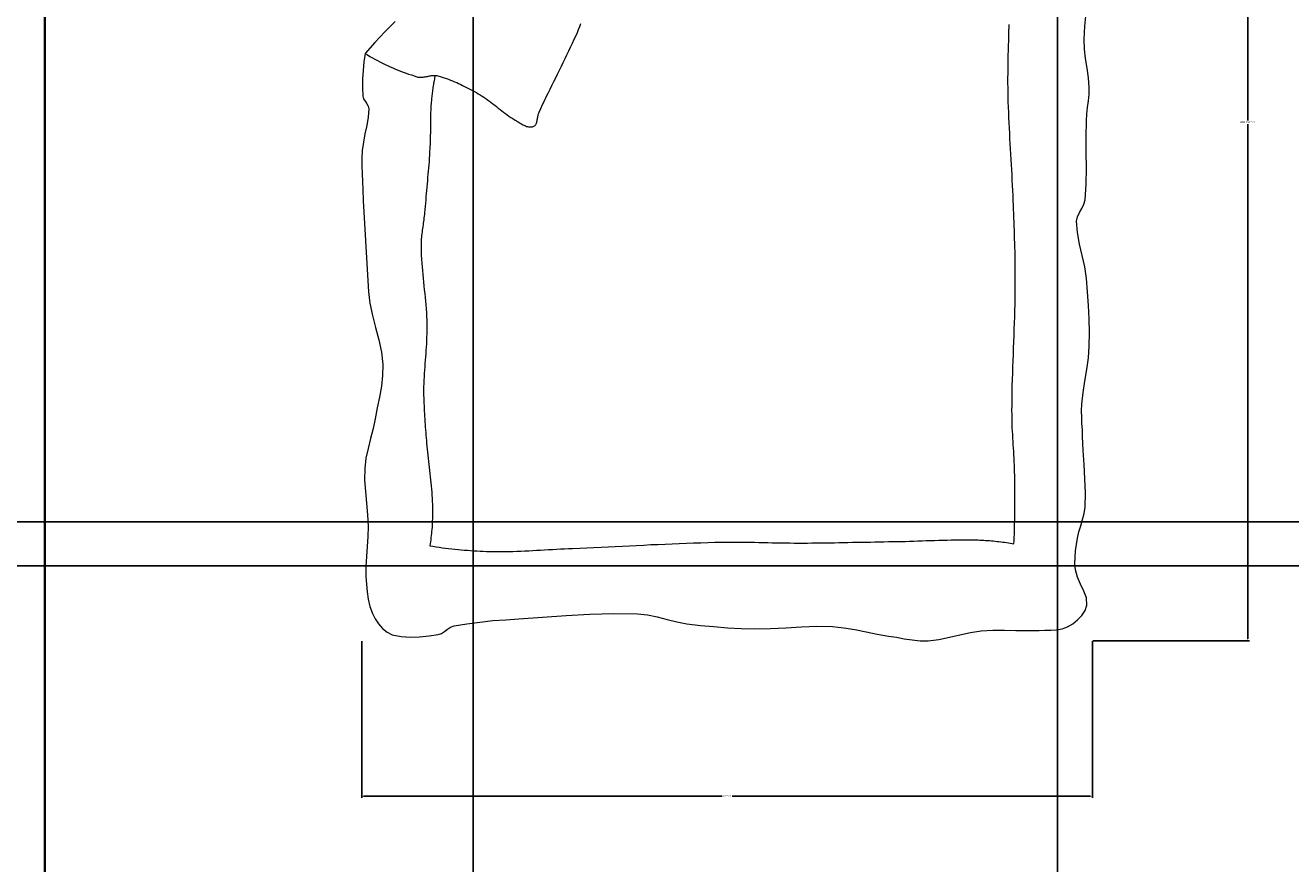
# Model space of a CAD drawing. Units: inches. Extents: x 1770 to 2988, y 1161 to 3221.
# Tile 13 of 44: x 2159 to 2289, y 2237 to 2323. Entities that reach past the tile are written whole.
import ezdxf

# ---------------------------------------------------------------- set-up
doc = ezdxf.new("R2010")
doc.units = ezdxf.units.IN
for name, color, linetype, lineweight in [('A-ANNO-DIMS', 2, 'Continuous', 18), ('A-FURN', 8, 'Continuous', 13), ('A-WALL', 7, 'Continuous', 35)]:
    doc.layers.add(name, color=color, linetype=linetype, lineweight=lineweight)
doc.styles.get("Standard").update_dxf_attribs({"font": 'arial.ttf'})
doc.dimstyles.get("Standard").update_dxf_attribs({"dimtxt": 0.18, "dimasz": 0.18, "dimexe": 0.18, "dimexo": 0.0625, "dimgap": 0.09, "dimtad": 0, "dimtih": 1, "dimtoh": 1, "dimdec": 4, "dimzin": 0, "dimdsep": 46, "dimtxsty": 'Standard', "dimcen": 0.09, "dimadec": 0, "dimazin": 0, "dimtfac": 1, "dimtdec": 4, "dimtofl": 0, "dimtmove": 0, "dimatfit": 3, "dimfxl": 1, "dimtolj": 1, "dimtzin": 0, "dimarcsym": 0})

# ---------------------------------------------------------------- blocks, each defined once
blk = doc.blocks.new('BED-DOUBLE-PLAN')
for p, q in [((74.2, 63.07), (74.35, 64.43)), ((2.36, 62.48), (1.33, 61.39)), ((3.42, 63.54), (2.36, 62.48)), ((21.99, 62.11), (22.12, 62.41)), ((22.12, 62.41), (22.25, 62.72)), ((22.25, 62.72), (22.37, 63.02)), ((22.37, 63.02), (22.49, 63.33)), ((66.41, 62.17), (66.42, 62.51)), ((66.42, 62.69), (66.43, 62.87)), ((66.42, 62.51), (66.42, 62.69)), ((66.43, 62.87), (66.44, 63.06)), ((66.44, 63.06), (66.45, 63.24)), ((74.12, 61.71), (74.2, 63.07)), ((1.33, 61.39), (0.33, 60.27)), ((21.43, 60.92), (21.62, 61.32)), ((21.62, 61.32), (21.8, 61.72)), ((21.8, 61.72), (21.99, 62.11)), ((66.37, 60.83), (66.38, 61.17)), ((66.38, 61.17), (66.39, 61.5)), ((66.39, 61.5), (66.4, 61.84)), ((66.4, 61.84), (66.41, 62.17)), ((74.16, 60.72), (74.12, 61.71)), ((0.33, 60.27), (0.2, 59.4)), ((0.33, 60.27), (0.58, 60.12)), ((0.58, 60.12), (0.83, 59.97)), ((0.83, 59.97), (1.08, 59.83)), ((1.08, 59.83), (1.34, 59.69)), ((20.86, 59.74), (21.05, 60.13)), ((21.05, 60.13), (21.24, 60.53)), ((21.24, 60.53), (21.43, 60.92)), ((66.34, 59.83), (66.35, 60.17)), ((66.34, 59.5), (66.34, 59.83)), ((66.35, 60.17), (66.36, 60.5)), ((66.36, 60.5), (66.37, 60.83)), ((74.28, 59.74), (74.16, 60.72)), ((0.12, 58.52), (0.07, 57.65)), ((0.2, 59.4), (0.12, 58.52)), ((1.34, 59.69), (1.6, 59.55)), ((1.6, 59.55), (1.85, 59.41)), ((1.85, 59.41), (2.11, 59.28)), ((2.11, 59.28), (2.38, 59.15)), ((2.38, 59.15), (2.64, 59.03)), ((2.64, 59.03), (2.91, 58.91)), ((2.91, 58.91), (3.17, 58.79)), ((3.17, 58.79), (3.44, 58.67)), ((3.44, 58.67), (3.71, 58.56)), ((3.71, 58.56), (3.98, 58.45)), ((3.98, 58.45), (4.25, 58.35)), ((20.09, 58.16), (20.29, 58.56)), ((20.29, 58.56), (20.48, 58.95)), ((20.48, 58.95), (20.67, 59.34)), ((20.67, 59.34), (20.86, 59.74)), ((66.32, 58.83), (66.33, 59.16)), ((66.32, 58.49), (66.32, 58.83)), ((66.32, 58.16), (66.32, 58.49)), ((66.33, 59.16), (66.34, 59.5)), ((74.44, 58.75), (74.28, 59.74)), ((74.58, 57.77), (74.44, 58.75)), ((0.07, 57.65), (0.07, 56.77)), ((4.25, 58.35), (4.53, 58.25)), ((4.53, 58.25), (4.8, 58.15)), ((4.8, 58.15), (5.08, 58.06)), ((5.08, 58.06), (5.35, 57.97)), ((5.35, 57.97), (5.63, 57.88)), ((5.63, 57.88), (5.73, 57.85)), ((5.73, 57.85), (5.84, 57.84)), ((5.84, 57.84), (5.95, 57.83)), ((5.95, 57.83), (6.06, 57.83)), ((6.06, 57.83), (6.17, 57.83)), ((6.17, 57.83), (6.28, 57.84)), ((6.28, 57.84), (6.39, 57.86)), ((6.39, 57.86), (6.5, 57.88)), ((6.5, 57.88), (6.61, 57.9)), ((6.61, 57.9), (6.72, 57.92)), ((6.72, 57.92), (6.83, 57.94)), ((6.83, 57.94), (6.94, 57.96)), ((6.94, 57.96), (7.05, 57.98)), ((7.05, 57.98), (7.16, 58)), ((7.16, 58), (7.27, 58.01)), ((7.27, 58.01), (7.38, 58.02)), ((7.36, 57.21), (7.34, 57.07)), ((7.39, 57.34), (7.36, 57.21)), ((7.38, 58.02), (7.49, 58.02)), ((7.41, 57.48), (7.39, 57.34)), ((7.44, 57.62), (7.41, 57.48)), ((7.47, 57.76), (7.44, 57.62)), ((7.5, 57.89), (7.47, 57.76)), ((7.49, 58.02), (7.6, 58.01)), ((7.6, 58.01), (7.71, 58)), ((7.71, 58), (7.81, 57.97)), ((7.81, 57.97), (8.03, 57.91)), ((8.03, 57.91), (8.25, 57.85)), ((8.25, 57.85), (8.46, 57.78)), ((8.46, 57.78), (8.67, 57.7)), ((8.67, 57.7), (8.89, 57.62)), ((8.89, 57.62), (9.1, 57.54)), ((9.1, 57.54), (9.31, 57.46)), ((9.31, 57.46), (9.52, 57.37)), ((9.52, 57.37), (9.73, 57.28)), ((9.73, 57.28), (9.93, 57.19)), ((9.93, 57.19), (10.14, 57.09)), ((19.51, 56.99), (19.71, 57.38)), ((19.71, 57.38), (19.9, 57.77)), ((19.9, 57.77), (20.09, 58.16)), ((66.31, 57.83), (66.32, 58.16)), ((66.31, 57.49), (66.31, 57.83)), ((66.31, 57.16), (66.31, 57.49)), ((66.32, 56.82), (66.31, 57.16)), ((74.65, 56.78), (74.58, 57.77)), ((0.07, 56.77), (0.11, 55.89)), ((0.11, 55.89), (0.18, 55.62)), ((7.19, 55.96), (7.17, 55.82)), ((7.2, 56.1), (7.19, 55.96)), ((7.22, 56.24), (7.2, 56.1)), ((7.24, 56.38), (7.22, 56.24)), ((7.25, 56.51), (7.24, 56.38)), ((7.27, 56.65), (7.25, 56.51)), ((7.3, 56.79), (7.27, 56.65)), ((7.32, 56.93), (7.3, 56.79)), ((7.34, 57.07), (7.32, 56.93)), ((10.14, 57.09), (10.34, 56.99)), ((10.34, 56.99), (10.55, 56.89)), ((10.55, 56.89), (10.75, 56.79)), ((10.75, 56.79), (10.95, 56.68)), ((10.95, 56.68), (11.15, 56.58)), ((11.15, 56.58), (11.35, 56.47)), ((11.35, 56.47), (11.55, 56.36)), ((11.55, 56.36), (11.75, 56.25)), ((11.75, 56.25), (11.94, 56.14)), ((11.94, 56.14), (12.14, 56.02)), ((12.14, 56.02), (12.33, 55.9)), ((12.33, 55.9), (12.53, 55.77)), ((18.93, 55.81), (19.13, 56.2)), ((19.13, 56.2), (19.32, 56.59)), ((19.32, 56.59), (19.51, 56.99)), ((66.32, 56.49), (66.32, 56.82)), ((66.32, 56.15), (66.32, 56.49)), ((66.33, 55.82), (66.32, 56.15)), ((74.58, 55.4), (74.64, 56.09)), ((74.64, 56.09), (74.65, 56.78)), ((0.18, 55.62), (0.34, 55.36)), ((0.34, 55.36), (0.51, 55.11)), ((0.51, 55.11), (0.66, 54.86)), ((0.72, 54.58), (0.65, 53.73)), ((0.66, 54.86), (0.72, 54.58)), ((7.08, 54.66), (7.07, 54.43)), ((7.09, 54.89), (7.08, 54.66)), ((7.11, 55.12), (7.09, 54.89)), ((7.12, 55.26), (7.11, 55.12)), ((7.13, 55.4), (7.12, 55.26)), ((7.14, 55.54), (7.13, 55.4)), ((7.16, 55.68), (7.14, 55.54)), ((7.17, 55.82), (7.16, 55.68)), ((12.53, 55.77), (12.71, 55.64)), ((12.71, 55.64), (12.9, 55.51)), ((12.9, 55.51), (13.09, 55.37)), ((13.09, 55.37), (13.27, 55.23)), ((13.27, 55.23), (13.45, 55.09)), ((13.45, 55.09), (13.63, 54.95)), ((13.63, 54.95), (13.82, 54.81)), ((13.82, 54.81), (14, 54.67)), ((14, 54.67), (14.18, 54.52)), ((18.18, 54.23), (18.36, 54.62)), ((18.36, 54.62), (18.55, 55.02)), ((18.55, 55.02), (18.74, 55.41)), ((18.74, 55.41), (18.93, 55.81)), ((66.35, 55.29), (66.33, 55.82)), ((66.37, 54.75), (66.35, 55.29)), ((66.39, 54.22), (66.37, 54.75)), ((74.41, 54.03), (74.49, 54.72)), ((74.49, 54.72), (74.58, 55.4)), ((0.65, 53.73), (0.5, 52.87)), ((7.05, 53.5), (7.04, 53.27)), ((7.04, 53.27), (7.04, 53.04)), ((7.06, 53.97), (7.05, 53.74)), ((7.05, 53.74), (7.05, 53.5)), ((7.07, 54.43), (7.06, 54.2)), ((7.06, 54.2), (7.06, 53.97)), ((14.18, 54.52), (14.36, 54.38)), ((14.36, 54.38), (14.54, 54.24)), ((14.54, 54.24), (14.73, 54.1)), ((14.73, 54.1), (14.91, 53.97)), ((14.91, 53.97), (15.1, 53.84)), ((15.1, 53.84), (15.29, 53.71)), ((15.29, 53.71), (15.48, 53.58)), ((15.48, 53.58), (15.68, 53.46)), ((15.68, 53.46), (15.77, 53.41)), ((15.77, 53.41), (15.86, 53.35)), ((15.86, 53.35), (15.95, 53.3)), ((15.95, 53.3), (16.04, 53.24)), ((17.95, 53.21), (17.97, 53.29)), ((17.97, 53.29), (17.99, 53.38)), ((17.99, 53.38), (18, 53.46)), ((18, 53.46), (18.02, 53.55)), ((18.02, 53.55), (18.03, 53.64)), ((18.03, 53.64), (18.05, 53.73)), ((18.05, 53.73), (18.06, 53.82)), ((18.06, 53.82), (18.08, 53.91)), ((18.08, 53.91), (18.1, 53.99)), ((18.1, 53.99), (18.12, 54.07)), ((18.12, 54.07), (18.15, 54.15)), ((18.15, 54.15), (18.18, 54.23)), ((66.41, 53.68), (66.39, 54.22)), ((66.43, 53.15), (66.41, 53.68)), ((74.34, 51.73), (74.36, 53.35)), ((74.36, 53.35), (74.41, 54.03)), ((0.32, 52.03), (0.15, 51.17)), ((0.5, 52.87), (0.32, 52.03)), ((7.03, 52.12), (7.02, 51.88)), ((7.04, 52.81), (7.03, 52.58)), ((7.03, 52.58), (7.03, 52.35)), ((7.03, 52.35), (7.03, 52.12)), ((7.04, 53.04), (7.04, 52.81)), ((16.04, 53.24), (16.13, 53.18)), ((16.13, 53.18), (16.23, 53.12)), ((16.23, 53.12), (16.32, 53.07)), ((16.32, 53.07), (16.42, 53.01)), ((16.42, 53.01), (16.51, 52.96)), ((16.51, 52.96), (16.61, 52.91)), ((16.61, 52.91), (16.71, 52.87)), ((16.71, 52.87), (16.81, 52.83)), ((16.81, 52.83), (16.9, 52.79)), ((16.9, 52.79), (17, 52.76)), ((17, 52.76), (17.1, 52.74)), ((17.1, 52.74), (17.2, 52.73)), ((17.2, 52.73), (17.3, 52.73)), ((17.3, 52.73), (17.4, 52.73)), ((17.4, 52.73), (17.5, 52.74)), ((17.5, 52.74), (17.59, 52.77)), ((17.59, 52.77), (17.66, 52.8)), ((17.66, 52.8), (17.73, 52.83)), ((17.73, 52.83), (17.78, 52.88)), ((17.78, 52.88), (17.82, 52.93)), ((17.82, 52.93), (17.86, 52.99)), ((17.86, 52.99), (17.9, 53.06)), ((17.9, 53.06), (17.93, 53.13)), ((17.93, 53.13), (17.95, 53.21)), ((66.46, 52.61), (66.43, 53.15)), ((66.49, 52.08), (66.46, 52.61)), ((66.52, 51.54), (66.49, 52.08)), ((0.15, 51.17), (0.04, 50.32)), ((6.99, 50.73), (6.97, 50.5)), ((7, 50.96), (6.99, 50.73)), ((7.01, 51.19), (7, 50.96)), ((7.02, 51.65), (7.01, 51.42)), ((7.01, 51.42), (7.01, 51.19)), ((7.02, 51.88), (7.02, 51.65)), ((66.55, 51.01), (66.52, 51.54)), ((66.58, 50.47), (66.55, 51.01)), ((74.35, 50.11), (74.34, 51.73)), ((0.04, 50.32), (0, 49.52)), ((0, 49.52), (0, 48.72)), ((6.91, 49.51), (6.89, 49.18)), ((6.93, 49.84), (6.91, 49.51)), ((6.95, 50.17), (6.93, 49.84)), ((6.97, 50.5), (6.95, 50.17)), ((66.61, 49.94), (66.58, 50.47)), ((66.64, 49.4), (66.61, 49.94)), ((66.67, 48.87), (66.64, 49.4)), ((74.36, 48.49), (74.35, 50.11)), ((0, 48.72), (0.02, 47.92)), ((6.81, 48.2), (6.78, 47.87)), ((6.84, 48.52), (6.81, 48.2)), ((6.86, 48.85), (6.84, 48.52)), ((6.89, 49.18), (6.86, 48.85)), ((66.7, 48.34), (66.67, 48.87)), ((66.73, 47.8), (66.7, 48.34)), ((74.34, 46.87), (74.36, 48.49)), ((0.02, 47.92), (0.06, 47.12)), ((0.06, 47.12), (0.09, 46.32)), ((6.7, 46.88), (6.67, 46.55)), ((6.73, 47.21), (6.7, 46.88)), ((6.75, 47.54), (6.73, 47.21)), ((6.78, 47.87), (6.75, 47.54)), ((66.76, 47.27), (66.73, 47.8)), ((66.79, 46.73), (66.76, 47.27)), ((74.23, 45.26), (74.34, 46.87)), ((0.09, 46.32), (0.14, 45.15)), ((6.58, 45.57), (6.55, 45.24)), ((6.61, 45.9), (6.58, 45.57)), ((6.64, 46.22), (6.61, 45.9)), ((6.67, 46.55), (6.64, 46.22)), ((66.82, 46.2), (66.79, 46.73)), ((66.84, 45.66), (66.82, 46.2)), ((66.86, 45.13), (66.84, 45.66)), ((0.14, 45.15), (0.2, 43.98)), ((6.46, 44.25), (6.43, 43.92)), ((6.49, 44.58), (6.46, 44.25)), ((6.52, 44.91), (6.49, 44.58)), ((6.55, 45.24), (6.52, 44.91)), ((66.88, 44.7), (66.86, 45.13)), ((66.89, 44.26), (66.88, 44.7)), ((66.91, 43.83), (66.89, 44.26)), ((73.64, 43.95), (73.89, 44.37)), ((73.89, 44.37), (74.11, 44.8)), ((74.11, 44.8), (74.23, 45.26)), ((0.2, 43.98), (0.26, 42.81)), ((6.33, 43.03), (6.3, 42.85)), ((6.35, 43.21), (6.33, 43.03)), ((6.37, 43.39), (6.35, 43.21)), ((6.4, 43.56), (6.37, 43.39)), ((6.42, 43.74), (6.4, 43.56)), ((6.43, 43.92), (6.42, 43.74)), ((66.93, 43.4), (66.91, 43.83)), ((66.94, 42.96), (66.93, 43.4)), ((66.96, 42.53), (66.94, 42.96)), ((73.36, 43.07), (73.44, 43.52)), ((73.46, 41.88), (73.36, 43.07)), ((73.44, 43.52), (73.64, 43.95)), ((0.26, 42.81), (0.33, 41.64)), ((0.33, 41.64), (0.4, 40.47)), ((6.13, 41.59), (6.11, 41.41)), ((6.15, 41.77), (6.13, 41.59)), ((6.18, 41.95), (6.15, 41.77)), ((6.2, 42.13), (6.18, 41.95)), ((6.22, 42.31), (6.2, 42.13)), ((6.25, 42.49), (6.22, 42.31)), ((6.28, 42.67), (6.25, 42.49)), ((6.3, 42.85), (6.28, 42.67)), ((66.97, 42.1), (66.96, 42.53)), ((66.99, 41.67), (66.97, 42.1)), ((67, 41.23), (66.99, 41.67)), ((73.67, 40.71), (73.46, 41.88)), ((0.4, 40.47), (0.47, 39.3)), ((6.08, 41.05), (6.07, 40.87)), ((6.07, 40.87), (6.07, 40.69)), ((6.07, 40.69), (6.07, 40.51)), ((6.07, 40.51), (6.07, 40.33)), ((6.07, 40.33), (6.08, 39.93)), ((6.1, 41.23), (6.08, 41.05)), ((6.11, 41.41), (6.1, 41.23)), ((67.01, 40.8), (67, 41.23)), ((67.03, 40.37), (67.01, 40.8)), ((67.04, 39.93), (67.03, 40.37)), ((73.93, 39.54), (73.67, 40.71)), ((0.47, 39.3), (0.53, 38.14)), ((6.08, 39.93), (6.1, 39.54)), ((6.1, 39.54), (6.12, 39.15)), ((6.12, 39.15), (6.15, 38.76)), ((67.05, 39.5), (67.04, 39.93)), ((67.05, 39.07), (67.05, 39.5)), ((67.06, 38.64), (67.05, 39.07)), ((74.19, 38.37), (73.93, 39.54)), ((0.53, 38.14), (0.6, 36.98)), ((6.15, 38.76), (6.18, 38.37)), ((6.18, 38.37), (6.21, 37.98)), ((6.21, 37.98), (6.25, 37.59)), ((67.07, 38.2), (67.06, 38.64)), ((67.07, 37.77), (67.07, 38.2)), ((67.07, 37.34), (67.07, 37.77)), ((74.37, 37.19), (74.19, 38.37)), ((0.6, 36.98), (0.69, 35.82)), ((6.25, 37.59), (6.29, 37.2)), ((6.29, 37.2), (6.33, 36.81)), ((6.33, 36.81), (6.37, 36.42)), ((6.37, 36.42), (6.41, 36.02)), ((67.07, 36.9), (67.07, 37.34)), ((67.07, 36.47), (67.07, 36.9)), ((67.07, 35.83), (67.07, 36.47)), ((74.49, 35.81), (74.37, 37.19)), ((0.69, 35.82), (0.83, 34.66)), ((6.41, 36.02), (6.45, 35.63)), ((6.45, 35.63), (6.49, 35.24)), ((6.49, 35.24), (6.53, 34.85)), ((67.04, 34.54), (67.06, 35.18)), ((67.06, 35.18), (67.07, 35.83)), ((74.59, 34.41), (74.49, 35.81)), ((0.83, 34.66), (1.08, 33.39)), ((6.53, 34.85), (6.56, 34.46)), ((6.56, 34.46), (6.59, 34.07)), ((6.59, 34.07), (6.62, 33.68)), ((67.01, 33.25), (67.03, 33.89)), ((67.03, 33.89), (67.04, 34.54)), ((74.66, 33.02), (74.59, 34.41)), ((1.08, 33.39), (1.4, 32.14)), ((6.62, 33.68), (6.64, 33.29)), ((6.64, 33.29), (6.66, 32.9)), ((6.66, 32.9), (6.67, 32.5)), ((6.67, 32.5), (6.67, 32.16)), ((66.96, 31.96), (66.99, 32.61)), ((66.99, 32.61), (67.01, 33.25)), ((74.68, 31.62), (74.66, 33.02)), ((1.4, 32.14), (1.73, 30.88)), ((6.66, 31.49), (6.65, 31.15)), ((6.67, 31.83), (6.66, 31.49)), ((6.67, 32.16), (6.67, 31.83)), ((66.92, 30.67), (66.94, 31.32)), ((66.94, 31.32), (66.96, 31.96)), ((74.66, 30.23), (74.68, 31.62)), ((1.73, 30.88), (2, 29.62)), ((6.6, 30.13), (6.57, 29.79)), ((6.62, 30.47), (6.6, 30.13)), ((6.64, 30.81), (6.62, 30.47)), ((6.65, 31.15), (6.64, 30.81)), ((66.87, 29.39), (66.89, 30.03)), ((66.89, 30.03), (66.92, 30.67)), ((74.57, 29.03), (74.66, 30.23)), ((2, 29.62), (2.14, 28.34)), ((6.5, 28.78), (6.47, 28.44)), ((6.52, 29.12), (6.5, 28.78)), ((6.55, 29.46), (6.52, 29.12)), ((6.57, 29.79), (6.55, 29.46)), ((66.82, 28.1), (66.84, 28.74)), ((66.84, 28.74), (66.87, 29.39)), ((74.4, 27.84), (74.57, 29.03)), ((2.14, 28.34), (2.12, 27.22)), ((6.4, 27.42), (6.38, 27.09)), ((6.42, 27.76), (6.4, 27.42)), ((6.45, 28.1), (6.42, 27.76)), ((6.47, 28.44), (6.45, 28.1)), ((66.78, 26.81), (66.8, 27.45)), ((66.8, 27.45), (66.82, 28.1)), ((74.21, 26.65), (74.4, 27.84)), ((2, 26.11), (1.8, 25)), ((2.12, 27.22), (2, 26.11)), ((6.35, 26.41), (6.34, 26.07)), ((6.34, 26.07), (6.34, 25.73)), ((6.36, 26.75), (6.35, 26.41)), ((6.38, 27.09), (6.36, 26.75)), ((66.75, 25.52), (66.76, 26.17)), ((66.76, 26.17), (66.78, 26.81)), ((74.03, 25.47), (74.21, 26.65)), ((1.8, 25), (1.58, 23.9)), ((6.34, 25.73), (6.34, 25.46)), ((6.34, 25.46), (6.34, 25.19)), ((6.34, 25.19), (6.35, 24.91)), ((6.35, 24.91), (6.36, 24.64)), ((66.73, 24.23), (66.74, 24.88)), ((66.74, 24.88), (66.75, 25.52)), ((73.9, 24.27), (74.03, 25.47)), ((1.58, 23.9), (1.37, 22.79)), ((6.36, 24.64), (6.36, 24.37)), ((6.36, 24.37), (6.38, 24.1)), ((6.38, 24.1), (6.39, 23.82)), ((6.39, 23.82), (6.4, 23.55)), ((6.4, 23.55), (6.42, 23.28)), ((66.72, 23.59), (66.73, 24.23)), ((66.73, 23.24), (66.72, 23.59)), ((73.87, 23.61), (73.9, 24.27)), ((73.88, 22.95), (73.87, 23.61)), ((1.37, 22.79), (1.15, 21.77)), ((6.42, 23.28), (6.43, 23.01)), ((6.43, 23.01), (6.45, 22.74)), ((6.45, 22.74), (6.47, 22.46)), ((6.47, 22.46), (6.49, 22.19)), ((6.49, 22.19), (6.51, 21.92)), ((66.73, 22.89), (66.73, 23.24)), ((66.74, 22.55), (66.73, 22.89)), ((66.75, 22.2), (66.74, 22.55)), ((66.76, 21.85), (66.75, 22.2)), ((73.91, 22.29), (73.88, 22.95)), ((73.95, 21.63), (73.91, 22.29)), ((1.15, 21.77), (0.89, 20.76)), ((6.51, 21.92), (6.53, 21.65)), ((6.53, 21.65), (6.55, 21.38)), ((6.55, 21.38), (6.57, 21.11)), ((6.57, 21.11), (6.59, 20.83)), ((6.59, 20.83), (6.62, 20.56)), ((66.78, 21.5), (66.76, 21.85)), ((66.8, 21.15), (66.78, 21.5)), ((66.82, 20.8), (66.8, 21.15)), ((66.84, 20.46), (66.82, 20.8)), ((73.98, 20.97), (73.95, 21.63)), ((74.05, 19.52), (73.98, 20.97)), ((0.64, 19.74), (0.42, 18.72)), ((0.89, 20.76), (0.64, 19.74)), ((6.62, 20.56), (6.64, 20.29)), ((6.64, 20.29), (6.66, 19.98)), ((6.66, 19.98), (6.69, 19.66)), ((6.69, 19.66), (6.72, 19.35)), ((66.86, 20.11), (66.84, 20.46)), ((66.88, 19.76), (66.86, 20.11)), ((66.9, 19.41), (66.88, 19.76)), ((74.14, 18.07), (74.05, 19.52)), ((0.42, 18.72), (0.3, 17.69)), ((6.72, 19.35), (6.76, 19.03)), ((6.76, 19.03), (6.79, 18.72)), ((6.79, 18.72), (6.83, 18.4)), ((6.83, 18.4), (6.86, 18.09)), ((66.92, 19.06), (66.9, 19.41)), ((66.94, 18.72), (66.92, 19.06)), ((66.96, 18.37), (66.94, 18.72)), ((66.97, 18.02), (66.96, 18.37)), ((0.3, 17.69), (0.28, 16.5)), ((6.86, 18.09), (6.9, 17.77)), ((6.9, 17.77), (6.94, 17.46)), ((6.94, 17.46), (6.98, 17.15)), ((6.98, 17.15), (7.01, 16.83)), ((66.99, 17.67), (66.97, 18.02)), ((67, 17.32), (66.99, 17.67)), ((67.01, 16.97), (67, 17.32)), ((67.02, 16.63), (67.01, 16.97)), ((74.22, 16.62), (74.14, 18.07)), ((0.28, 16.5), (0.36, 15.3)), ((7.01, 16.83), (7.05, 16.52)), ((7.05, 16.52), (7.08, 16.2)), ((7.08, 16.2), (7.11, 15.89)), ((7.11, 15.89), (7.14, 15.57)), ((67.02, 16.29), (67.02, 16.63)), ((67.03, 15.96), (67.02, 16.29)), ((67.03, 15.62), (67.03, 15.96)), ((67.03, 15.29), (67.03, 15.62)), ((74.26, 15.17), (74.22, 16.62)), ((0.36, 15.3), (0.48, 14.11)), ((7.14, 15.57), (7.17, 15.26)), ((7.17, 15.26), (7.19, 14.94)), ((7.19, 14.94), (7.21, 14.63)), ((7.21, 14.63), (7.23, 14.31)), ((7.23, 14.31), (7.24, 13.99)), ((67.03, 14.95), (67.03, 15.29)), ((67.03, 14.62), (67.03, 14.95)), ((67.03, 14.29), (67.03, 14.62)), ((74.24, 13.72), (74.26, 15.17)), ((0.48, 14.11), (0.59, 12.92)), ((7.24, 13.99), (7.25, 13.78)), ((7.25, 13.78), (7.25, 13.57)), ((7.25, 13.57), (7.26, 13.35)), ((7.26, 13.14), (7.25, 12.93)), ((7.26, 13.35), (7.26, 13.14)), ((67.02, 13.28), (67.03, 13.62)), ((67.02, 12.95), (67.02, 13.28)), ((67.03, 13.95), (67.03, 14.29)), ((67.03, 13.62), (67.03, 13.95)), ((73.98, 12.43), (74.15, 13.07)), ((74.15, 13.07), (74.24, 13.72)), ((0.59, 12.92), (0.65, 11.72)), ((0.65, 11.72), (0.62, 10.69)), ((7.21, 11.86), (7.2, 11.65)), ((7.22, 12.07), (7.21, 11.86)), ((7.23, 12.29), (7.22, 12.07)), ((7.24, 12.5), (7.23, 12.29)), ((7.25, 12.71), (7.24, 12.5)), ((7.25, 12.93), (7.25, 12.71)), ((66.99, 11.61), (67, 11.95)), ((67, 11.95), (67.01, 12.28)), ((67.01, 12.61), (67.02, 12.95)), ((67.01, 12.28), (67.01, 12.61)), ((73.59, 11.17), (73.78, 11.8)), ((73.78, 11.8), (73.98, 12.43)), ((0.62, 10.69), (0.55, 9.66)), ((7.09, 10.58), (7.07, 10.37)), ((7.12, 10.8), (7.09, 10.58)), ((7.14, 11.01), (7.12, 10.8)), ((7.16, 11.22), (7.14, 11.01)), ((7.18, 11.43), (7.16, 11.22)), ((7.2, 11.65), (7.18, 11.43)), ((66.95, 10.27), (66.96, 10.61)), ((66.96, 10.61), (66.97, 10.94)), ((66.97, 10.94), (66.98, 11.28)), ((66.98, 11.28), (66.99, 11.61)), ((73.35, 9.87), (73.45, 10.52)), ((73.45, 10.52), (73.59, 11.17)), ((0.55, 9.66), (0.47, 8.63)), ((7.01, 9.95), (6.98, 9.74)), ((6.98, 9.74), (7.3, 9.69)), ((7.04, 10.16), (7.01, 9.95)), ((7.07, 10.37), (7.04, 10.16)), ((7.3, 9.69), (7.62, 9.64)), ((7.62, 9.64), (7.94, 9.59)), ((7.94, 9.59), (8.26, 9.55)), ((8.26, 9.55), (8.58, 9.5)), ((8.58, 9.5), (8.9, 9.47)), ((8.9, 9.47), (9.22, 9.43)), ((9.22, 9.43), (9.55, 9.39)), ((9.55, 9.39), (9.87, 9.36)), ((9.87, 9.36), (10.19, 9.33)), ((10.19, 9.33), (10.51, 9.3)), ((10.51, 9.3), (10.84, 9.28)), ((10.84, 9.28), (11.16, 9.25)), ((11.16, 9.25), (11.48, 9.23)), ((11.48, 9.23), (11.81, 9.21)), ((11.81, 9.21), (12.13, 9.2)), ((12.13, 9.2), (12.45, 9.18)), ((12.45, 9.18), (12.78, 9.17)), ((12.78, 9.17), (13.1, 9.16)), ((13.1, 9.16), (13.43, 9.15)), ((13.43, 9.15), (13.84, 9.15)), ((13.84, 9.15), (14.25, 9.15)), ((14.25, 9.15), (14.66, 9.15)), ((14.66, 9.15), (15.07, 9.16)), ((15.07, 9.16), (15.48, 9.17)), ((15.48, 9.17), (15.89, 9.18)), ((15.89, 9.18), (16.3, 9.2)), ((16.3, 9.2), (16.71, 9.21)), ((16.71, 9.21), (17.12, 9.23)), ((17.12, 9.23), (17.53, 9.25)), ((17.53, 9.25), (17.94, 9.28)), ((17.94, 9.28), (18.35, 9.3)), ((18.35, 9.3), (18.76, 9.32)), ((18.76, 9.32), (19.17, 9.35)), ((19.17, 9.35), (19.58, 9.37)), ((19.58, 9.37), (19.99, 9.4)), ((19.99, 9.4), (20.4, 9.42)), ((20.4, 9.42), (20.81, 9.44)), ((20.81, 9.44), (21.22, 9.46)), ((21.22, 9.46), (21.63, 9.48)), ((21.63, 9.48), (22.36, 9.51)), ((22.36, 9.51), (23.09, 9.54)), ((23.09, 9.54), (23.82, 9.57)), ((23.82, 9.57), (24.55, 9.61)), ((24.55, 9.61), (25.28, 9.64)), ((25.28, 9.64), (26.01, 9.68)), ((26.01, 9.68), (26.74, 9.72)), ((26.74, 9.72), (27.47, 9.75)), ((27.47, 9.75), (28.2, 9.79)), ((28.2, 9.79), (28.93, 9.82)), ((28.93, 9.82), (29.66, 9.86)), ((29.66, 9.86), (30.39, 9.89)), ((30.39, 9.89), (31.12, 9.92)), ((31.12, 9.92), (31.85, 9.95)), ((31.85, 9.95), (32.58, 9.98)), ((32.58, 9.98), (33.31, 10.01)), ((33.31, 10.01), (34.04, 10.04)), ((34.04, 10.04), (34.78, 10.06)), ((34.78, 10.06), (35.51, 10.08)), ((35.51, 10.08), (36.24, 10.1)), ((36.24, 10.1), (36.69, 10.11)), ((36.69, 10.11), (37.14, 10.12)), ((37.14, 10.12), (37.59, 10.12)), ((37.59, 10.12), (38.04, 10.12)), ((38.04, 10.12), (38.5, 10.12)), ((38.5, 10.12), (38.95, 10.11)), ((38.95, 10.11), (39.4, 10.11)), ((39.4, 10.11), (39.85, 10.1)), ((39.85, 10.1), (40.3, 10.1)), ((40.3, 10.1), (40.75, 10.09)), ((40.75, 10.09), (41.21, 10.08)), ((41.21, 10.08), (41.66, 10.07)), ((41.66, 10.07), (42.11, 10.06)), ((42.11, 10.06), (42.56, 10.05)), ((42.56, 10.05), (43.01, 10.05)), ((43.01, 10.05), (43.47, 10.04)), ((43.47, 10.04), (43.92, 10.04)), ((43.92, 10.04), (44.37, 10.03)), ((44.37, 10.03), (44.82, 10.03)), ((44.82, 10.03), (45.27, 10.03)), ((45.27, 10.03), (45.74, 10.03)), ((45.74, 10.03), (46.2, 10.04)), ((46.2, 10.04), (46.66, 10.04)), ((46.66, 10.04), (47.12, 10.05)), ((47.12, 10.05), (47.58, 10.05)), ((47.58, 10.05), (48.04, 10.06)), ((48.04, 10.06), (48.51, 10.06)), ((48.51, 10.06), (48.97, 10.07)), ((48.97, 10.07), (49.43, 10.08)), ((49.43, 10.08), (49.89, 10.09)), ((49.89, 10.09), (50.35, 10.1)), ((50.35, 10.1), (50.82, 10.1)), ((50.82, 10.1), (51.28, 10.11)), ((51.28, 10.11), (51.74, 10.12)), ((51.74, 10.12), (52.2, 10.13)), ((52.2, 10.13), (52.66, 10.14)), ((52.66, 10.14), (53.12, 10.15)), ((53.12, 10.15), (53.59, 10.16)), ((53.59, 10.16), (54.05, 10.17)), ((54.05, 10.17), (54.51, 10.17)), ((54.51, 10.17), (54.94, 10.18)), ((54.94, 10.18), (55.36, 10.19)), ((55.36, 10.19), (55.79, 10.2)), ((55.79, 10.2), (56.22, 10.22)), ((56.22, 10.22), (56.64, 10.23)), ((56.64, 10.23), (57.07, 10.24)), ((57.07, 10.24), (57.5, 10.26)), ((57.5, 10.26), (57.92, 10.27)), ((57.92, 10.27), (58.35, 10.28)), ((58.35, 10.28), (58.78, 10.3)), ((58.78, 10.3), (59.21, 10.31)), ((59.21, 10.31), (59.63, 10.32)), ((59.63, 10.32), (60.06, 10.33)), ((60.06, 10.33), (60.49, 10.34)), ((60.49, 10.34), (60.91, 10.34)), ((60.91, 10.34), (61.34, 10.35)), ((61.34, 10.35), (61.77, 10.35)), ((61.77, 10.35), (62.19, 10.35)), ((62.19, 10.35), (62.62, 10.35)), ((62.62, 10.35), (63.05, 10.34)), ((63.05, 10.34), (63.24, 10.34)), ((63.24, 10.34), (63.44, 10.33)), ((63.44, 10.33), (63.63, 10.32)), ((63.63, 10.32), (63.83, 10.31)), ((63.83, 10.31), (64.02, 10.3)), ((64.02, 10.3), (64.22, 10.29)), ((64.22, 10.29), (64.41, 10.28)), ((64.41, 10.28), (64.61, 10.26)), ((64.61, 10.26), (64.8, 10.24)), ((64.8, 10.24), (65, 10.22)), ((65, 10.22), (65.19, 10.2)), ((65.19, 10.2), (65.39, 10.18)), ((65.39, 10.18), (65.58, 10.15)), ((65.58, 10.15), (65.78, 10.13)), ((65.78, 10.13), (65.97, 10.1)), ((65.97, 10.1), (66.16, 10.07)), ((66.16, 10.07), (66.36, 10.04)), ((66.36, 10.04), (66.55, 10.01)), ((66.55, 10.01), (66.74, 9.98)), ((66.74, 9.98), (66.93, 9.94)), ((66.93, 9.94), (66.95, 10.27)), ((73.2, 8.56), (73.26, 9.22)), ((73.26, 9.22), (73.35, 9.87)), ((0.47, 8.63), (0.41, 7.61)), ((73.19, 7.91), (73.2, 8.56)), ((73.24, 7.26), (73.19, 7.91)), ((0.41, 7.61), (0.42, 6.58)), ((0.42, 6.58), (0.47, 5.81)), ((73.44, 6.52), (73.24, 7.26)), ((73.77, 5.81), (73.44, 6.52)), ((0.47, 5.81), (0.53, 5.03)), ((74.11, 5.1), (73.77, 5.81)), ((0.53, 5.03), (0.65, 4.26)), ((0.65, 4.26), (0.82, 3.52)), ((74.36, 4.39), (74.11, 5.1)), ((74.4, 3.66), (74.36, 4.39)), ((0.82, 3.52), (1.09, 2.8)), ((1.09, 2.8), (1.37, 2.25)), ((20.98, 2.58), (23.41, 2.71)), ((23.41, 2.71), (25.85, 2.78)), ((25.85, 2.78), (28.28, 2.76)), ((28.28, 2.76), (29.3, 2.66)), ((29.3, 2.66), (30.32, 2.45)), ((73.9, 2.58), (74.23, 3.09)), ((74.23, 3.09), (74.4, 3.66)), ((1.37, 2.25), (1.71, 1.73)), ((1.71, 1.73), (2.12, 1.26)), ((8.8, 1.19), (9.11, 1.39)), ((9.11, 1.39), (9.46, 1.52)), ((9.46, 1.52), (10.78, 1.74)), ((10.78, 1.74), (12.11, 1.92)), ((12.11, 1.92), (13.44, 2.06)), ((13.44, 2.06), (14.78, 2.16)), ((14.78, 2.16), (16.12, 2.26)), ((16.12, 2.26), (18.55, 2.42)), ((18.55, 2.42), (20.98, 2.58)), ((30.32, 2.45), (31.33, 2.18)), ((31.33, 2.18), (32.34, 1.93)), ((32.34, 1.93), (33.36, 1.75)), ((33.36, 1.75), (34.75, 1.58)), ((34.75, 1.58), (36.14, 1.45)), ((36.14, 1.45), (37.54, 1.34)), ((37.54, 1.34), (38.94, 1.26)), ((41.93, 1.24), (43.52, 1.32)), ((43.52, 1.32), (45.12, 1.42)), ((45.12, 1.42), (46.71, 1.48)), ((46.71, 1.48), (48.3, 1.45)), ((48.3, 1.45), (49.46, 1.34)), ((49.46, 1.34), (50.61, 1.15)), ((71.89, 1.21), (72.43, 1.42)), ((72.43, 1.42), (72.96, 1.74)), ((72.96, 1.74), (73.46, 2.13)), ((73.46, 2.13), (73.9, 2.58)), ((2.12, 1.26), (2.59, 0.88)), ((2.59, 0.88), (3.12, 0.62)), ((3.12, 0.62), (4.04, 0.42)), ((4.04, 0.42), (4.98, 0.36)), ((4.98, 0.36), (5.93, 0.41)), ((5.93, 0.41), (6.89, 0.52)), ((6.89, 0.52), (7.83, 0.65)), ((7.83, 0.65), (8.17, 0.76)), ((8.17, 0.76), (8.49, 0.96)), ((8.49, 0.96), (8.8, 1.19)), ((38.94, 1.26), (40.34, 1.22)), ((40.34, 1.22), (41.93, 1.24)), ((50.61, 1.15), (51.76, 0.91)), ((51.76, 0.91), (52.9, 0.68)), ((52.9, 0.68), (54.06, 0.48)), ((54.06, 0.48), (54.86, 0.35)), ((54.86, 0.35), (55.67, 0.2)), ((55.67, 0.2), (56.48, 0.08)), ((56.48, 0.08), (57.3, 0)), ((57.3, 0), (58.11, 0)), ((58.11, 0), (59.21, 0.13)), ((59.21, 0.13), (60.3, 0.35)), ((60.3, 0.35), (61.39, 0.6)), ((61.39, 0.6), (62.47, 0.84)), ((62.47, 0.84), (63.57, 1)), ((63.57, 1), (64.76, 1.07)), ((64.76, 1.07), (65.95, 1.07)), ((65.95, 1.07), (67.13, 1.05)), ((67.13, 1.05), (68.32, 1.04)), ((68.32, 1.04), (69.51, 1.06)), ((69.51, 1.06), (70.11, 1.07)), ((70.11, 1.07), (70.71, 1.08)), ((70.71, 1.08), (71.31, 1.11)), ((71.31, 1.11), (71.89, 1.21))]:
    blk.add_line(p, q)
blk = doc.blocks.new('*D38')
at = {"layer": 'A-ANNO-DIMS', "color": 0, "lineweight": -2, "transparency": 16777216}
for p, q in [((2268.29, 2365.92), (2284.37, 2365.92)), ((2284.19, 2365.74), (2284.19, 2312.89)), ((2284.19, 2259.68), (2284.19, 2312.52)), ((2268.29, 2259.5), (2284.37, 2259.5))]:
    blk.add_line(p, q, dxfattribs=at)
at = {"layer": 'A-ANNO-DIMS', "color": 0, "transparency": 16777216}
for points in [[(2284.16, 2365.74), (2284.22, 2365.74), (2284.19, 2365.92)], [(2284.16, 2259.68), (2284.22, 2259.68), (2284.19, 2259.5)]]:
    blk.add_solid(points, dxfattribs=at)
at = {"layer": 'Defpoints', "color": 0, "transparency": 16777216}
for p in [(2268.23, 2365.92), (2284.19, 2365.92), (2268.23, 2259.5)]:
    blk.add_point(p, dxfattribs=at)
at = {"layer": 'A-ANNO-DIMS', "color": 0, "transparency": 16777216, "insert": (2284.19, 2312.71), "char_height": 0.18, "attachment_point": 5}
blk.add_mtext('\\A1;BED 106 TYP.', dxfattribs=at)
blk = doc.blocks.new('*D39')
at = {"layer": 'A-ANNO-DIMS', "color": 0, "lineweight": -2, "transparency": 16777216}
for p, q in [((2193.25, 2259.44), (2193.25, 2243.36)), ((2268.23, 2259.44), (2268.23, 2243.36)), ((2193.43, 2243.54), (2230.22, 2243.54)), ((2268.05, 2243.54), (2231.27, 2243.54))]:
    blk.add_line(p, q, dxfattribs=at)
at = {"layer": 'A-ANNO-DIMS', "color": 0, "transparency": 16777216}
for points in [[(2193.43, 2243.57), (2193.43, 2243.51), (2193.25, 2243.54)], [(2268.05, 2243.57), (2268.05, 2243.51), (2268.23, 2243.54)]]:
    blk.add_solid(points, dxfattribs=at)
at = {"layer": 'Defpoints', "color": 0, "transparency": 16777216}
for p in [(2193.25, 2259.5), (2268.23, 2259.5), (2268.23, 2243.54)]:
    blk.add_point(p, dxfattribs=at)
at = {"layer": 'A-ANNO-DIMS', "color": 0, "transparency": 16777216, "insert": (2230.74, 2243.54), "char_height": 0.18, "attachment_point": 5}
blk.add_mtext('\\A1;75 TYP.', dxfattribs=at)
blk = doc.blocks.new('*D72')
at = {"layer": 'A-ANNO-DIMS', "color": 0, "lineweight": -2, "transparency": 16777216}
for p, q in [((2456.13, 2267.2), (1907.1, 2267.2)), ((1907.28, 2267.02), (1907.28, 2221.63)), ((1907.28, 2175.88), (1907.28, 2221.27)), ((2456.13, 2175.7), (1907.1, 2175.7))]:
    blk.add_line(p, q, dxfattribs=at)
at = {"layer": 'A-ANNO-DIMS', "color": 0, "transparency": 16777216}
for points in [[(1907.25, 2267.02), (1907.31, 2267.02), (1907.28, 2267.2)], [(1907.25, 2175.88), (1907.31, 2175.88), (1907.28, 2175.7)]]:
    blk.add_solid(points, dxfattribs=at)
at = {"layer": 'Defpoints', "color": 0, "transparency": 16777216}
for p in [(1907.28, 2267.2), (2456.2, 2267.2), (2456.2, 2175.7)]:
    blk.add_point(p, dxfattribs=at)
at = {"layer": 'A-ANNO-DIMS', "color": 0, "transparency": 16777216, "insert": (1907.28, 2221.45), "char_height": 0.18, "attachment_point": 5}
blk.add_mtext('\\A1;91.5', dxfattribs=at)
blk = doc.blocks.new('*D73')
at = {"layer": 'A-ANNO-DIMS', "color": 0, "lineweight": -2, "transparency": 16777216}
for p, q in [((2456.13, 2367.7), (1907.1, 2367.7)), ((1907.28, 2367.52), (1907.28, 2319.88)), ((1907.28, 2271.88), (1907.28, 2319.52)), ((2456.13, 2271.7), (1907.1, 2271.7))]:
    blk.add_line(p, q, dxfattribs=at)
at = {"layer": 'A-ANNO-DIMS', "color": 0, "transparency": 16777216}
for points in [[(1907.25, 2367.52), (1907.31, 2367.52), (1907.28, 2367.7)], [(1907.25, 2271.88), (1907.31, 2271.88), (1907.28, 2271.7)]]:
    blk.add_solid(points, dxfattribs=at)
at = {"layer": 'Defpoints', "color": 0, "transparency": 16777216}
for p in [(1907.28, 2367.7), (2456.2, 2367.7), (2456.2, 2271.7)]:
    blk.add_point(p, dxfattribs=at)
at = {"layer": 'A-ANNO-DIMS', "color": 0, "transparency": 16777216, "insert": (1907.28, 2319.7), "char_height": 0.18, "attachment_point": 5}
blk.add_mtext('\\A1;96', dxfattribs=at)
blk = doc.blocks.new('*D79')
at = {"layer": 'A-ANNO-DIMS', "color": 0, "lineweight": -2, "transparency": 16777216}
for p, q in [((2151.7, 1610.26), (2151.7, 2570.7)), ((2151.88, 2570.52), (2177.78, 2570.52)), ((2204.48, 2570.52), (2178.57, 2570.52)), ((2204.66, 1610.26), (2204.66, 2570.7))]:
    blk.add_line(p, q, dxfattribs=at)
at = {"layer": 'A-ANNO-DIMS', "color": 0, "transparency": 16777216}
for points in [[(2151.88, 2570.55), (2151.88, 2570.49), (2151.7, 2570.52)], [(2204.48, 2570.55), (2204.48, 2570.49), (2204.66, 2570.52)]]:
    blk.add_solid(points, dxfattribs=at)
at = {"layer": 'Defpoints', "color": 0, "transparency": 16777216}
for p in [(2204.66, 2570.52), (2151.7, 1610.2), (2204.66, 1610.2)]:
    blk.add_point(p, dxfattribs=at)
at = {"layer": 'A-ANNO-DIMS', "color": 0, "transparency": 16777216, "insert": (2178.18, 2570.52), "char_height": 0.18, "attachment_point": 5}
blk.add_mtext('\\A1;52.96', dxfattribs=at)
blk = doc.blocks.new('*D80')
at = {"layer": 'A-ANNO-DIMS', "color": 0, "lineweight": -2, "transparency": 16777216}
for p, q in [((2264.66, 1610.26), (2264.66, 2570.7)), ((2264.84, 2570.52), (2314.14, 2570.52)), ((2364.23, 2570.52), (2314.93, 2570.52)), ((2364.41, 1610.26), (2364.41, 2570.7))]:
    blk.add_line(p, q, dxfattribs=at)
at = {"layer": 'A-ANNO-DIMS', "color": 0, "transparency": 16777216}
for points in [[(2264.84, 2570.55), (2264.84, 2570.49), (2264.66, 2570.52)], [(2364.23, 2570.55), (2364.23, 2570.49), (2364.41, 2570.52)]]:
    blk.add_solid(points, dxfattribs=at)
at = {"layer": 'Defpoints', "color": 0, "transparency": 16777216}
for p in [(2364.41, 2570.52), (2264.66, 1610.2), (2364.41, 1610.2)]:
    blk.add_point(p, dxfattribs=at)
at = {"layer": 'A-ANNO-DIMS', "color": 0, "transparency": 16777216, "insert": (2314.53, 2570.52), "char_height": 0.18, "attachment_point": 5}
blk.add_mtext('\\A1;99.76', dxfattribs=at)

msp = doc.modelspace()

# ---------------------------------------------------------------- linework, layer by layer
at = {"layer": 'A-WALL'}
msp.add_line((2160.696, 2367.7021), (2160.696, 2175.7021), dxfattribs=at)

# ---------------------------------------------------------------- block references
at = {"layer": 'A-FURN'}
msp.add_blockref('BED-DOUBLE-PLAN', (2193.254, 2259.498), dxfattribs=at)

# ---------------------------------------------------------------- dimensions: what is measured, and where the dimension line sits
at = {"layer": 'A-ANNO-DIMS'}
for base, p1, p2, picture, middle in [((2204.6568, 2570.5247), (2151.696, 1610.2021), (2204.6568, 1610.2021), '*D79', (2178.1764, 2570.5247)), ((2364.4122, 2570.5247), (2264.6568, 1610.2021), (2364.4122, 1610.2021), '*D80', (2314.5345, 2570.5247))]:
    dim = msp.add_linear_dim(base=base, p1=p1, p2=p2, dimstyle='Standard', override={"dimdec": 2, "dimlfac": 1, "dimrnd": 0, "dimzin": 0, "dimdsep": 46, "dimlunit": 2}, dxfattribs=at)
    dim.commit()
    dim.dimension.update_dxf_attribs({"geometry": picture, "text_midpoint": middle})
for base, p1, p2, override, picture, middle in [((1907.2844, 2367.7021), (2456.196, 2271.7021), (2456.196, 2367.7021), {"dimdec": 0, "dimlfac": 1, "dimrnd": 0, "dimzin": 0, "dimdsep": 46, "dimlunit": 2}, '*D73', (1907.2844, 2319.7021)), ((1907.2844, 2267.2021), (2456.196, 2175.7021), (2456.196, 2267.2021), {"dimdec": 1, "dimlfac": 1, "dimrnd": 0, "dimzin": 0, "dimdsep": 46, "dimlunit": 2}, '*D72', (1907.2844, 2221.4521))]:
    dim = msp.add_linear_dim(base=base, p1=p1, p2=p2, angle=90, dimstyle='Standard', override=override, dxfattribs=at)
    dim.commit()
    dim.dimension.update_dxf_attribs({"geometry": picture, "text_midpoint": middle})
dim = msp.add_linear_dim(base=(2284.1945, 2365.9152), p1=(2268.232, 2259.4983), p2=(2268.232, 2365.9152), angle=90, text='BED <> TYP.', dimstyle='Standard', override={"dimdec": 0, "dimlfac": 1, "dimrnd": 0, "dimzin": 0, "dimdsep": 46, "dimlunit": 2}, dxfattribs=at)
dim.commit()
dim.dimension.update_dxf_attribs({"geometry": '*D38', "text_midpoint": (2284.1945, 2312.7068)})
dim = msp.add_linear_dim(base=(2268.232, 2243.5358), p1=(2193.2538, 2259.4983), p2=(2268.232, 2259.4983), text='<> TYP.', dimstyle='Standard', override={"dimdec": 0, "dimlfac": 1, "dimrnd": 0, "dimzin": 0, "dimdsep": 46, "dimlunit": 2}, dxfattribs=at)
dim.commit()
dim.dimension.update_dxf_attribs({"geometry": '*D39', "text_midpoint": (2230.7429, 2243.5358)})

doc.saveas('drawing.dxf')
